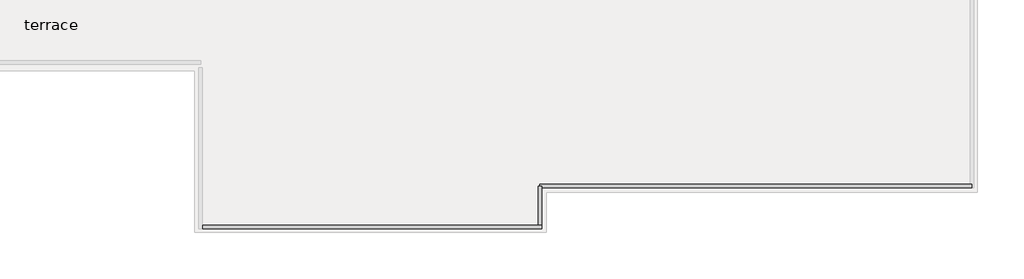
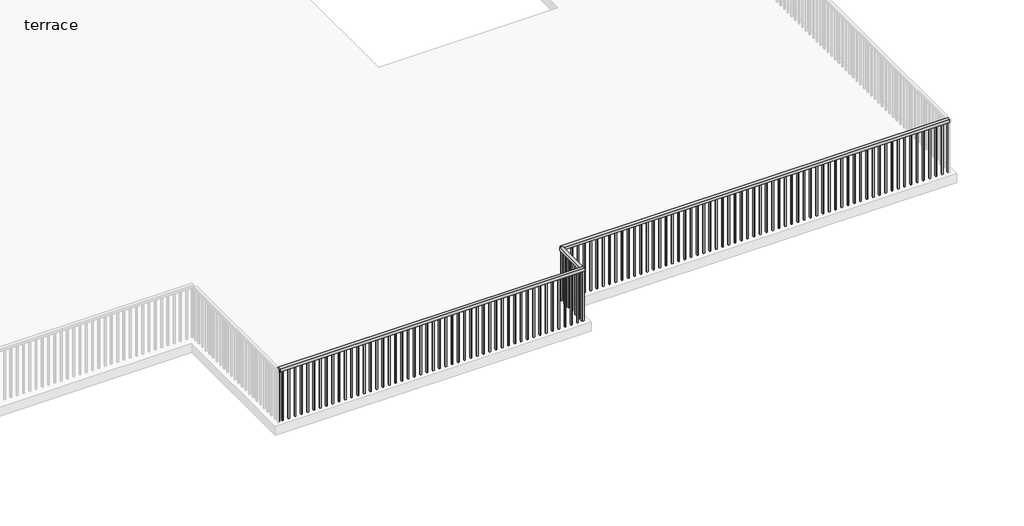
# One storey, part 2 of 7: 3 railings.
"""IFC4 building model written with IfcOpenShell, lengths in millimetres."""

from ifc_helpers import new_model, si_unit, frame, origin, place, context, project, spatial, polyline, outline, extrude, element, save

model = new_model("IFC4")

# Units and contexts
model_context = context("Model", 3, world=origin())
ifc_project = project(units=[si_unit("LENGTHUNIT", "METRE", prefix="MILLI")], contexts=[model_context])

# Site, building, storey
site = spatial("IfcSite", under=ifc_project)
building = spatial("IfcBuilding", under=site)
storey = spatial("IfcBuildingStorey", under=building, Name="terrace", Elevation=3810.0)

# Railings
placement = place(None, origin())
element("IfcRailing", 1, ObjectType="Handrail - Rectangular", at=placement, inside=storey, context=model_context, shape_type="SweptSolid", body=[
    extrude(outline(polyline([(1292.9109871, -4498.672378), (1292.9109871, -4549.472378), (-4974.5390129, -4549.472378), (-4974.5390129, -4498.672378), (1292.9109871, -4498.672378)])), frame((0.0, 0.0, 4673.6), z_axis=(0.0, 0.0, 1.0), x_axis=(1.0, 0.0, 0.0)), (0.0, 0.0, 1.0), 50.8),
    extrude(outline(polyline([(-4895.1640129, -4514.547378), (-4895.1640129, -4533.597378), (-4914.2140129, -4533.597378), (-4914.2140129, -4514.547378), (-4895.1640129, -4514.547378)])), frame((0.0, 0.0, 3810.0), z_axis=(0.0, 0.0, 1.0), x_axis=(1.0, 0.0, 0.0)), (0.0, 0.0, 1.0), 863.6),
    extrude(outline(polyline([(-4793.5640129, -4514.547378), (-4793.5640129, -4533.597378), (-4812.6140129, -4533.597378), (-4812.6140129, -4514.547378), (-4793.5640129, -4514.547378)])), frame((0.0, 0.0, 3810.0), z_axis=(0.0, 0.0, 1.0), x_axis=(1.0, 0.0, 0.0)), (0.0, 0.0, 1.0), 863.6),
    extrude(outline(polyline([(-4691.9640129, -4514.547378), (-4691.9640129, -4533.597378), (-4711.0140129, -4533.597378), (-4711.0140129, -4514.547378), (-4691.9640129, -4514.547378)])), frame((0.0, 0.0, 3810.0), z_axis=(0.0, 0.0, 1.0), x_axis=(1.0, 0.0, 0.0)), (0.0, 0.0, 1.0), 863.6),
    extrude(outline(polyline([(-4590.3640129, -4514.547378), (-4590.3640129, -4533.597378), (-4609.4140129, -4533.597378), (-4609.4140129, -4514.547378), (-4590.3640129, -4514.547378)])), frame((0.0, 0.0, 3810.0), z_axis=(0.0, 0.0, 1.0), x_axis=(1.0, 0.0, 0.0)), (0.0, 0.0, 1.0), 863.6),
    extrude(outline(polyline([(-4488.7640129, -4514.547378), (-4488.7640129, -4533.597378), (-4507.8140129, -4533.597378), (-4507.8140129, -4514.547378), (-4488.7640129, -4514.547378)])), frame((0.0, 0.0, 3810.0), z_axis=(0.0, 0.0, 1.0), x_axis=(1.0, 0.0, 0.0)), (0.0, 0.0, 1.0), 863.6),
    extrude(outline(polyline([(-4387.1640129, -4514.547378), (-4387.1640129, -4533.597378), (-4406.2140129, -4533.597378), (-4406.2140129, -4514.547378), (-4387.1640129, -4514.547378)])), frame((0.0, 0.0, 3810.0), z_axis=(0.0, 0.0, 1.0), x_axis=(1.0, 0.0, 0.0)), (0.0, 0.0, 1.0), 863.6),
    extrude(outline(polyline([(-4285.5640129, -4514.547378), (-4285.5640129, -4533.597378), (-4304.6140129, -4533.597378), (-4304.6140129, -4514.547378), (-4285.5640129, -4514.547378)])), frame((0.0, 0.0, 3810.0), z_axis=(0.0, 0.0, 1.0), x_axis=(1.0, 0.0, 0.0)), (0.0, 0.0, 1.0), 863.6),
    extrude(outline(polyline([(-4183.9640129, -4514.547378), (-4183.9640129, -4533.597378), (-4203.0140129, -4533.597378), (-4203.0140129, -4514.547378), (-4183.9640129, -4514.547378)])), frame((0.0, 0.0, 3810.0), z_axis=(0.0, 0.0, 1.0), x_axis=(1.0, 0.0, 0.0)), (0.0, 0.0, 1.0), 863.6),
    extrude(outline(polyline([(-4082.3640129, -4514.547378), (-4082.3640129, -4533.597378), (-4101.4140129, -4533.597378), (-4101.4140129, -4514.547378), (-4082.3640129, -4514.547378)])), frame((0.0, 0.0, 3810.0), z_axis=(0.0, 0.0, 1.0), x_axis=(1.0, 0.0, 0.0)), (0.0, 0.0, 1.0), 863.6),
    extrude(outline(polyline([(-3980.7640129, -4514.547378), (-3980.7640129, -4533.597378), (-3999.8140129, -4533.597378), (-3999.8140129, -4514.547378), (-3980.7640129, -4514.547378)])), frame((0.0, 0.0, 3810.0), z_axis=(0.0, 0.0, 1.0), x_axis=(1.0, 0.0, 0.0)), (0.0, 0.0, 1.0), 863.6),
    extrude(outline(polyline([(-3879.1640129, -4514.547378), (-3879.1640129, -4533.597378), (-3898.2140129, -4533.597378), (-3898.2140129, -4514.547378), (-3879.1640129, -4514.547378)])), frame((0.0, 0.0, 3810.0), z_axis=(0.0, 0.0, 1.0), x_axis=(1.0, 0.0, 0.0)), (0.0, 0.0, 1.0), 863.6),
    extrude(outline(polyline([(-3777.5640129, -4514.547378), (-3777.5640129, -4533.597378), (-3796.6140129, -4533.597378), (-3796.6140129, -4514.547378), (-3777.5640129, -4514.547378)])), frame((0.0, 0.0, 3810.0), z_axis=(0.0, 0.0, 1.0), x_axis=(1.0, 0.0, 0.0)), (0.0, 0.0, 1.0), 863.6),
    extrude(outline(polyline([(-3675.9640129, -4514.547378), (-3675.9640129, -4533.597378), (-3695.0140129, -4533.597378), (-3695.0140129, -4514.547378), (-3675.9640129, -4514.547378)])), frame((0.0, 0.0, 3810.0), z_axis=(0.0, 0.0, 1.0), x_axis=(1.0, 0.0, 0.0)), (0.0, 0.0, 1.0), 863.6),
    extrude(outline(polyline([(-3574.3640129, -4514.547378), (-3574.3640129, -4533.597378), (-3593.4140129, -4533.597378), (-3593.4140129, -4514.547378), (-3574.3640129, -4514.547378)])), frame((0.0, 0.0, 3810.0), z_axis=(0.0, 0.0, 1.0), x_axis=(1.0, 0.0, 0.0)), (0.0, 0.0, 1.0), 863.6),
    extrude(outline(polyline([(-3472.7640129, -4514.547378), (-3472.7640129, -4533.597378), (-3491.8140129, -4533.597378), (-3491.8140129, -4514.547378), (-3472.7640129, -4514.547378)])), frame((0.0, 0.0, 3810.0), z_axis=(0.0, 0.0, 1.0), x_axis=(1.0, 0.0, 0.0)), (0.0, 0.0, 1.0), 863.6),
    extrude(outline(polyline([(-3371.1640129, -4514.547378), (-3371.1640129, -4533.597378), (-3390.2140129, -4533.597378), (-3390.2140129, -4514.547378), (-3371.1640129, -4514.547378)])), frame((0.0, 0.0, 3810.0), z_axis=(0.0, 0.0, 1.0), x_axis=(1.0, 0.0, 0.0)), (0.0, 0.0, 1.0), 863.6),
    extrude(outline(polyline([(-3269.5640129, -4514.547378), (-3269.5640129, -4533.597378), (-3288.6140129, -4533.597378), (-3288.6140129, -4514.547378), (-3269.5640129, -4514.547378)])), frame((0.0, 0.0, 3810.0), z_axis=(0.0, 0.0, 1.0), x_axis=(1.0, 0.0, 0.0)), (0.0, 0.0, 1.0), 863.6),
    extrude(outline(polyline([(-3167.9640129, -4514.547378), (-3167.9640129, -4533.597378), (-3187.0140129, -4533.597378), (-3187.0140129, -4514.547378), (-3167.9640129, -4514.547378)])), frame((0.0, 0.0, 3810.0), z_axis=(0.0, 0.0, 1.0), x_axis=(1.0, 0.0, 0.0)), (0.0, 0.0, 1.0), 863.6),
    extrude(outline(polyline([(-3066.3640129, -4514.547378), (-3066.3640129, -4533.597378), (-3085.4140129, -4533.597378), (-3085.4140129, -4514.547378), (-3066.3640129, -4514.547378)])), frame((0.0, 0.0, 3810.0), z_axis=(0.0, 0.0, 1.0), x_axis=(1.0, 0.0, 0.0)), (0.0, 0.0, 1.0), 863.6),
    extrude(outline(polyline([(-2964.7640129, -4514.547378), (-2964.7640129, -4533.597378), (-2983.8140129, -4533.597378), (-2983.8140129, -4514.547378), (-2964.7640129, -4514.547378)])), frame((0.0, 0.0, 3810.0), z_axis=(0.0, 0.0, 1.0), x_axis=(1.0, 0.0, 0.0)), (0.0, 0.0, 1.0), 863.6),
    extrude(outline(polyline([(-2863.1640129, -4514.547378), (-2863.1640129, -4533.597378), (-2882.2140129, -4533.597378), (-2882.2140129, -4514.547378), (-2863.1640129, -4514.547378)])), frame((0.0, 0.0, 3810.0), z_axis=(0.0, 0.0, 1.0), x_axis=(1.0, 0.0, 0.0)), (0.0, 0.0, 1.0), 863.6),
    extrude(outline(polyline([(-2761.5640129, -4514.547378), (-2761.5640129, -4533.597378), (-2780.6140129, -4533.597378), (-2780.6140129, -4514.547378), (-2761.5640129, -4514.547378)])), frame((0.0, 0.0, 3810.0), z_axis=(0.0, 0.0, 1.0), x_axis=(1.0, 0.0, 0.0)), (0.0, 0.0, 1.0), 863.6),
    extrude(outline(polyline([(-2659.9640129, -4514.547378), (-2659.9640129, -4533.597378), (-2679.0140129, -4533.597378), (-2679.0140129, -4514.547378), (-2659.9640129, -4514.547378)])), frame((0.0, 0.0, 3810.0), z_axis=(0.0, 0.0, 1.0), x_axis=(1.0, 0.0, 0.0)), (0.0, 0.0, 1.0), 863.6),
    extrude(outline(polyline([(-2558.3640129, -4514.547378), (-2558.3640129, -4533.597378), (-2577.4140129, -4533.597378), (-2577.4140129, -4514.547378), (-2558.3640129, -4514.547378)])), frame((0.0, 0.0, 3810.0), z_axis=(0.0, 0.0, 1.0), x_axis=(1.0, 0.0, 0.0)), (0.0, 0.0, 1.0), 863.6),
    extrude(outline(polyline([(-2456.7640129, -4514.547378), (-2456.7640129, -4533.597378), (-2475.8140129, -4533.597378), (-2475.8140129, -4514.547378), (-2456.7640129, -4514.547378)])), frame((0.0, 0.0, 3810.0), z_axis=(0.0, 0.0, 1.0), x_axis=(1.0, 0.0, 0.0)), (0.0, 0.0, 1.0), 863.6),
    extrude(outline(polyline([(-2355.1640129, -4514.547378), (-2355.1640129, -4533.597378), (-2374.2140129, -4533.597378), (-2374.2140129, -4514.547378), (-2355.1640129, -4514.547378)])), frame((0.0, 0.0, 3810.0), z_axis=(0.0, 0.0, 1.0), x_axis=(1.0, 0.0, 0.0)), (0.0, 0.0, 1.0), 863.6),
    extrude(outline(polyline([(-2253.5640129, -4514.547378), (-2253.5640129, -4533.597378), (-2272.6140129, -4533.597378), (-2272.6140129, -4514.547378), (-2253.5640129, -4514.547378)])), frame((0.0, 0.0, 3810.0), z_axis=(0.0, 0.0, 1.0), x_axis=(1.0, 0.0, 0.0)), (0.0, 0.0, 1.0), 863.6),
    extrude(outline(polyline([(-2151.9640129, -4514.547378), (-2151.9640129, -4533.597378), (-2171.0140129, -4533.597378), (-2171.0140129, -4514.547378), (-2151.9640129, -4514.547378)])), frame((0.0, 0.0, 3810.0), z_axis=(0.0, 0.0, 1.0), x_axis=(1.0, 0.0, 0.0)), (0.0, 0.0, 1.0), 863.6),
    extrude(outline(polyline([(-2050.3640129, -4514.547378), (-2050.3640129, -4533.597378), (-2069.4140129, -4533.597378), (-2069.4140129, -4514.547378), (-2050.3640129, -4514.547378)])), frame((0.0, 0.0, 3810.0), z_axis=(0.0, 0.0, 1.0), x_axis=(1.0, 0.0, 0.0)), (0.0, 0.0, 1.0), 863.6),
    extrude(outline(polyline([(-1948.7640129, -4514.547378), (-1948.7640129, -4533.597378), (-1967.8140129, -4533.597378), (-1967.8140129, -4514.547378), (-1948.7640129, -4514.547378)])), frame((0.0, 0.0, 3810.0), z_axis=(0.0, 0.0, 1.0), x_axis=(1.0, 0.0, 0.0)), (0.0, 0.0, 1.0), 863.6),
    extrude(outline(polyline([(-1847.1640129, -4514.547378), (-1847.1640129, -4533.597378), (-1866.2140129, -4533.597378), (-1866.2140129, -4514.547378), (-1847.1640129, -4514.547378)])), frame((0.0, 0.0, 3810.0), z_axis=(0.0, 0.0, 1.0), x_axis=(1.0, 0.0, 0.0)), (0.0, 0.0, 1.0), 863.6),
    extrude(outline(polyline([(-1745.5640129, -4514.547378), (-1745.5640129, -4533.597378), (-1764.6140129, -4533.597378), (-1764.6140129, -4514.547378), (-1745.5640129, -4514.547378)])), frame((0.0, 0.0, 3810.0), z_axis=(0.0, 0.0, 1.0), x_axis=(1.0, 0.0, 0.0)), (0.0, 0.0, 1.0), 863.6),
    extrude(outline(polyline([(-1643.9640129, -4514.547378), (-1643.9640129, -4533.597378), (-1663.0140129, -4533.597378), (-1663.0140129, -4514.547378), (-1643.9640129, -4514.547378)])), frame((0.0, 0.0, 3810.0), z_axis=(0.0, 0.0, 1.0), x_axis=(1.0, 0.0, 0.0)), (0.0, 0.0, 1.0), 863.6),
    extrude(outline(polyline([(-1542.3640129, -4514.547378), (-1542.3640129, -4533.597378), (-1561.4140129, -4533.597378), (-1561.4140129, -4514.547378), (-1542.3640129, -4514.547378)])), frame((0.0, 0.0, 3810.0), z_axis=(0.0, 0.0, 1.0), x_axis=(1.0, 0.0, 0.0)), (0.0, 0.0, 1.0), 863.6),
    extrude(outline(polyline([(-1440.7640129, -4514.547378), (-1440.7640129, -4533.597378), (-1459.8140129, -4533.597378), (-1459.8140129, -4514.547378), (-1440.7640129, -4514.547378)])), frame((0.0, 0.0, 3810.0), z_axis=(0.0, 0.0, 1.0), x_axis=(1.0, 0.0, 0.0)), (0.0, 0.0, 1.0), 863.6),
    extrude(outline(polyline([(-1339.1640129, -4514.547378), (-1339.1640129, -4533.597378), (-1358.2140129, -4533.597378), (-1358.2140129, -4514.547378), (-1339.1640129, -4514.547378)])), frame((0.0, 0.0, 3810.0), z_axis=(0.0, 0.0, 1.0), x_axis=(1.0, 0.0, 0.0)), (0.0, 0.0, 1.0), 863.6),
    extrude(outline(polyline([(-1237.5640129, -4514.547378), (-1237.5640129, -4533.597378), (-1256.6140129, -4533.597378), (-1256.6140129, -4514.547378), (-1237.5640129, -4514.547378)])), frame((0.0, 0.0, 3810.0), z_axis=(0.0, 0.0, 1.0), x_axis=(1.0, 0.0, 0.0)), (0.0, 0.0, 1.0), 863.6),
    extrude(outline(polyline([(-1135.9640129, -4514.547378), (-1135.9640129, -4533.597378), (-1155.0140129, -4533.597378), (-1155.0140129, -4514.547378), (-1135.9640129, -4514.547378)])), frame((0.0, 0.0, 3810.0), z_axis=(0.0, 0.0, 1.0), x_axis=(1.0, 0.0, 0.0)), (0.0, 0.0, 1.0), 863.6),
    extrude(outline(polyline([(-1034.3640129, -4514.547378), (-1034.3640129, -4533.597378), (-1053.4140129, -4533.597378), (-1053.4140129, -4514.547378), (-1034.3640129, -4514.547378)])), frame((0.0, 0.0, 3810.0), z_axis=(0.0, 0.0, 1.0), x_axis=(1.0, 0.0, 0.0)), (0.0, 0.0, 1.0), 863.6),
    extrude(outline(polyline([(-932.7640129, -4514.547378), (-932.7640129, -4533.597378), (-951.8140129, -4533.597378), (-951.8140129, -4514.547378), (-932.7640129, -4514.547378)])), frame((0.0, 0.0, 3810.0), z_axis=(0.0, 0.0, 1.0), x_axis=(1.0, 0.0, 0.0)), (0.0, 0.0, 1.0), 863.6),
    extrude(outline(polyline([(-831.1640129, -4514.547378), (-831.1640129, -4533.597378), (-850.2140129, -4533.597378), (-850.2140129, -4514.547378), (-831.1640129, -4514.547378)])), frame((0.0, 0.0, 3810.0), z_axis=(0.0, 0.0, 1.0), x_axis=(1.0, 0.0, 0.0)), (0.0, 0.0, 1.0), 863.6),
    extrude(outline(polyline([(-729.5640129, -4514.547378), (-729.5640129, -4533.597378), (-748.6140129, -4533.597378), (-748.6140129, -4514.547378), (-729.5640129, -4514.547378)])), frame((0.0, 0.0, 3810.0), z_axis=(0.0, 0.0, 1.0), x_axis=(1.0, 0.0, 0.0)), (0.0, 0.0, 1.0), 863.6),
    extrude(outline(polyline([(-627.9640129, -4514.547378), (-627.9640129, -4533.597378), (-647.0140129, -4533.597378), (-647.0140129, -4514.547378), (-627.9640129, -4514.547378)])), frame((0.0, 0.0, 3810.0), z_axis=(0.0, 0.0, 1.0), x_axis=(1.0, 0.0, 0.0)), (0.0, 0.0, 1.0), 863.6),
    extrude(outline(polyline([(-526.3640129, -4514.547378), (-526.3640129, -4533.597378), (-545.4140129, -4533.597378), (-545.4140129, -4514.547378), (-526.3640129, -4514.547378)])), frame((0.0, 0.0, 3810.0), z_axis=(0.0, 0.0, 1.0), x_axis=(1.0, 0.0, 0.0)), (0.0, 0.0, 1.0), 863.6),
    extrude(outline(polyline([(-424.7640129, -4514.547378), (-424.7640129, -4533.597378), (-443.8140129, -4533.597378), (-443.8140129, -4514.547378), (-424.7640129, -4514.547378)])), frame((0.0, 0.0, 3810.0), z_axis=(0.0, 0.0, 1.0), x_axis=(1.0, 0.0, 0.0)), (0.0, 0.0, 1.0), 863.6),
    extrude(outline(polyline([(-323.1640129, -4514.547378), (-323.1640129, -4533.597378), (-342.2140129, -4533.597378), (-342.2140129, -4514.547378), (-323.1640129, -4514.547378)])), frame((0.0, 0.0, 3810.0), z_axis=(0.0, 0.0, 1.0), x_axis=(1.0, 0.0, 0.0)), (0.0, 0.0, 1.0), 863.6),
    extrude(outline(polyline([(-221.5640129, -4514.547378), (-221.5640129, -4533.597378), (-240.6140129, -4533.597378), (-240.6140129, -4514.547378), (-221.5640129, -4514.547378)])), frame((0.0, 0.0, 3810.0), z_axis=(0.0, 0.0, 1.0), x_axis=(1.0, 0.0, 0.0)), (0.0, 0.0, 1.0), 863.6),
    extrude(outline(polyline([(-119.9640129, -4514.547378), (-119.9640129, -4533.597378), (-139.0140129, -4533.597378), (-139.0140129, -4514.547378), (-119.9640129, -4514.547378)])), frame((0.0, 0.0, 3810.0), z_axis=(0.0, 0.0, 1.0), x_axis=(1.0, 0.0, 0.0)), (0.0, 0.0, 1.0), 863.6),
    extrude(outline(polyline([(-18.3640129, -4514.547378), (-18.3640129, -4533.597378), (-37.4140129, -4533.597378), (-37.4140129, -4514.547378), (-18.3640129, -4514.547378)])), frame((0.0, 0.0, 3810.0), z_axis=(0.0, 0.0, 1.0), x_axis=(1.0, 0.0, 0.0)), (0.0, 0.0, 1.0), 863.6),
    extrude(outline(polyline([(83.2359871, -4514.547378), (83.2359871, -4533.597378), (64.1859871, -4533.597378), (64.1859871, -4514.547378), (83.2359871, -4514.547378)])), frame((0.0, 0.0, 3810.0), z_axis=(0.0, 0.0, 1.0), x_axis=(1.0, 0.0, 0.0)), (0.0, 0.0, 1.0), 863.6),
    extrude(outline(polyline([(184.8359871, -4514.547378), (184.8359871, -4533.597378), (165.7859871, -4533.597378), (165.7859871, -4514.547378), (184.8359871, -4514.547378)])), frame((0.0, 0.0, 3810.0), z_axis=(0.0, 0.0, 1.0), x_axis=(1.0, 0.0, 0.0)), (0.0, 0.0, 1.0), 863.6),
    extrude(outline(polyline([(286.4359871, -4514.547378), (286.4359871, -4533.597378), (267.3859871, -4533.597378), (267.3859871, -4514.547378), (286.4359871, -4514.547378)])), frame((0.0, 0.0, 3810.0), z_axis=(0.0, 0.0, 1.0), x_axis=(1.0, 0.0, 0.0)), (0.0, 0.0, 1.0), 863.6),
    extrude(outline(polyline([(388.0359871, -4514.547378), (388.0359871, -4533.597378), (368.9859871, -4533.597378), (368.9859871, -4514.547378), (388.0359871, -4514.547378)])), frame((0.0, 0.0, 3810.0), z_axis=(0.0, 0.0, 1.0), x_axis=(1.0, 0.0, 0.0)), (0.0, 0.0, 1.0), 863.6),
    extrude(outline(polyline([(489.6359871, -4514.547378), (489.6359871, -4533.597378), (470.5859871, -4533.597378), (470.5859871, -4514.547378), (489.6359871, -4514.547378)])), frame((0.0, 0.0, 3810.0), z_axis=(0.0, 0.0, 1.0), x_axis=(1.0, 0.0, 0.0)), (0.0, 0.0, 1.0), 863.6),
    extrude(outline(polyline([(591.2359871, -4514.547378), (591.2359871, -4533.597378), (572.1859871, -4533.597378), (572.1859871, -4514.547378), (591.2359871, -4514.547378)])), frame((0.0, 0.0, 3810.0), z_axis=(0.0, 0.0, 1.0), x_axis=(1.0, 0.0, 0.0)), (0.0, 0.0, 1.0), 863.6),
    extrude(outline(polyline([(692.8359871, -4514.547378), (692.8359871, -4533.597378), (673.7859871, -4533.597378), (673.7859871, -4514.547378), (692.8359871, -4514.547378)])), frame((0.0, 0.0, 3810.0), z_axis=(0.0, 0.0, 1.0), x_axis=(1.0, 0.0, 0.0)), (0.0, 0.0, 1.0), 863.6),
    extrude(outline(polyline([(794.4359871, -4514.547378), (794.4359871, -4533.597378), (775.3859871, -4533.597378), (775.3859871, -4514.547378), (794.4359871, -4514.547378)])), frame((0.0, 0.0, 3810.0), z_axis=(0.0, 0.0, 1.0), x_axis=(1.0, 0.0, 0.0)), (0.0, 0.0, 1.0), 863.6),
    extrude(outline(polyline([(896.0359871, -4514.547378), (896.0359871, -4533.597378), (876.9859871, -4533.597378), (876.9859871, -4514.547378), (896.0359871, -4514.547378)])), frame((0.0, 0.0, 3810.0), z_axis=(0.0, 0.0, 1.0), x_axis=(1.0, 0.0, 0.0)), (0.0, 0.0, 1.0), 863.6),
    extrude(outline(polyline([(997.6359871, -4514.547378), (997.6359871, -4533.597378), (978.5859871, -4533.597378), (978.5859871, -4514.547378), (997.6359871, -4514.547378)])), frame((0.0, 0.0, 3810.0), z_axis=(0.0, 0.0, 1.0), x_axis=(1.0, 0.0, 0.0)), (0.0, 0.0, 1.0), 863.6),
    extrude(outline(polyline([(1099.2359871, -4514.547378), (1099.2359871, -4533.597378), (1080.1859871, -4533.597378), (1080.1859871, -4514.547378), (1099.2359871, -4514.547378)])), frame((0.0, 0.0, 3810.0), z_axis=(0.0, 0.0, 1.0), x_axis=(1.0, 0.0, 0.0)), (0.0, 0.0, 1.0), 863.6),
    extrude(outline(polyline([(1200.8359871, -4514.547378), (1200.8359871, -4533.597378), (1181.7859871, -4533.597378), (1181.7859871, -4514.547378), (1200.8359871, -4514.547378)])), frame((0.0, 0.0, 3810.0), z_axis=(0.0, 0.0, 1.0), x_axis=(1.0, 0.0, 0.0)), (0.0, 0.0, 1.0), 863.6),
    extrude(outline(polyline([(-4955.4890129, -4514.547378), (-4955.4890129, -4533.597378), (-4974.5390129, -4533.597378), (-4974.5390129, -4514.547378), (-4955.4890129, -4514.547378)])), frame((0.0, 0.0, 3810.0), z_axis=(0.0, 0.0, 1.0), x_axis=(1.0, 0.0, 0.0)), (0.0, 0.0, 1.0), 863.6),
    extrude(outline(polyline([(1292.9109871, -4514.547378), (1292.9109871, -4533.597378), (1273.8609871, -4533.597378), (1273.8609871, -4514.547378), (1292.9109871, -4514.547378)])), frame((0.0, 0.0, 3810.0), z_axis=(0.0, 0.0, 1.0), x_axis=(1.0, 0.0, 0.0)), (0.0, 0.0, 1.0), 863.6),
])
element("IfcRailing", 2, ObjectType="Handrail - Rectangular", at=placement, inside=storey, context=model_context, shape_type="SweptSolid", body=[
    extrude(outline(polyline([(-4999.9390129, -4524.072378), (-4949.1390129, -4524.072378), (-4949.1390129, -5114.622378), (-4999.9390129, -5114.622378), (-4999.9390129, -4524.072378)])), frame((0.0, 0.0, 4673.6), z_axis=(0.0, 0.0, 1.0), x_axis=(1.0, 0.0, 0.0)), (0.0, 0.0, 1.0), 50.8),
    extrude(outline(polyline([(-4984.0640129, -5022.547378), (-4965.0140129, -5022.547378), (-4965.0140129, -5041.597378), (-4984.0640129, -5041.597378), (-4984.0640129, -5022.547378)])), frame((0.0, 0.0, 3810.0), z_axis=(0.0, 0.0, 1.0), x_axis=(1.0, 0.0, 0.0)), (0.0, 0.0, 1.0), 863.6),
    extrude(outline(polyline([(-4984.0640129, -4920.947378), (-4965.0140129, -4920.947378), (-4965.0140129, -4939.997378), (-4984.0640129, -4939.997378), (-4984.0640129, -4920.947378)])), frame((0.0, 0.0, 3810.0), z_axis=(0.0, 0.0, 1.0), x_axis=(1.0, 0.0, 0.0)), (0.0, 0.0, 1.0), 863.6),
    extrude(outline(polyline([(-4984.0640129, -4819.347378), (-4965.0140129, -4819.347378), (-4965.0140129, -4838.397378), (-4984.0640129, -4838.397378), (-4984.0640129, -4819.347378)])), frame((0.0, 0.0, 3810.0), z_axis=(0.0, 0.0, 1.0), x_axis=(1.0, 0.0, 0.0)), (0.0, 0.0, 1.0), 863.6),
    extrude(outline(polyline([(-4984.0640129, -4717.747378), (-4965.0140129, -4717.747378), (-4965.0140129, -4736.797378), (-4984.0640129, -4736.797378), (-4984.0640129, -4717.747378)])), frame((0.0, 0.0, 3810.0), z_axis=(0.0, 0.0, 1.0), x_axis=(1.0, 0.0, 0.0)), (0.0, 0.0, 1.0), 863.6),
    extrude(outline(polyline([(-4984.0640129, -4616.147378), (-4965.0140129, -4616.147378), (-4965.0140129, -4635.197378), (-4984.0640129, -4635.197378), (-4984.0640129, -4616.147378)])), frame((0.0, 0.0, 3810.0), z_axis=(0.0, 0.0, 1.0), x_axis=(1.0, 0.0, 0.0)), (0.0, 0.0, 1.0), 863.6),
    extrude(outline(polyline([(-4984.0640129, -5095.572378), (-4965.0140129, -5095.572378), (-4965.0140129, -5114.622378), (-4984.0640129, -5114.622378), (-4984.0640129, -5095.572378)])), frame((0.0, 0.0, 3810.0), z_axis=(0.0, 0.0, 1.0), x_axis=(1.0, 0.0, 0.0)), (0.0, 0.0, 1.0), 863.6),
    extrude(outline(polyline([(-4984.0640129, -4524.072378), (-4965.0140129, -4524.072378), (-4965.0140129, -4543.122378), (-4984.0640129, -4543.122378), (-4984.0640129, -4524.072378)])), frame((0.0, 0.0, 3810.0), z_axis=(0.0, 0.0, 1.0), x_axis=(1.0, 0.0, 0.0)), (0.0, 0.0, 1.0), 863.6),
])
element("IfcRailing", 3, ObjectType="Handrail - Rectangular", at=placement, inside=storey, context=model_context, shape_type="SweptSolid", body=[
    extrude(outline(polyline([(-4949.1390129, -5089.222378), (-4949.1390129, -5140.022378), (-9895.7890129, -5140.022378), (-9895.7890129, -5089.222378), (-4949.1390129, -5089.222378)])), frame((0.0, 0.0, 4673.6), z_axis=(0.0, 0.0, 1.0), x_axis=(1.0, 0.0, 0.0)), (0.0, 0.0, 1.0), 50.8),
    extrude(outline(polyline([(-9816.4140129, -5105.097378), (-9816.4140129, -5124.147378), (-9835.4640129, -5124.147378), (-9835.4640129, -5105.097378), (-9816.4140129, -5105.097378)])), frame((0.0, 0.0, 3810.0), z_axis=(0.0, 0.0, 1.0), x_axis=(1.0, 0.0, 0.0)), (0.0, 0.0, 1.0), 863.6),
    extrude(outline(polyline([(-9714.8140129, -5105.097378), (-9714.8140129, -5124.147378), (-9733.8640129, -5124.147378), (-9733.8640129, -5105.097378), (-9714.8140129, -5105.097378)])), frame((0.0, 0.0, 3810.0), z_axis=(0.0, 0.0, 1.0), x_axis=(1.0, 0.0, 0.0)), (0.0, 0.0, 1.0), 863.6),
    extrude(outline(polyline([(-9613.2140129, -5105.097378), (-9613.2140129, -5124.147378), (-9632.2640129, -5124.147378), (-9632.2640129, -5105.097378), (-9613.2140129, -5105.097378)])), frame((0.0, 0.0, 3810.0), z_axis=(0.0, 0.0, 1.0), x_axis=(1.0, 0.0, 0.0)), (0.0, 0.0, 1.0), 863.6),
    extrude(outline(polyline([(-9511.6140129, -5105.097378), (-9511.6140129, -5124.147378), (-9530.6640129, -5124.147378), (-9530.6640129, -5105.097378), (-9511.6140129, -5105.097378)])), frame((0.0, 0.0, 3810.0), z_axis=(0.0, 0.0, 1.0), x_axis=(1.0, 0.0, 0.0)), (0.0, 0.0, 1.0), 863.6),
    extrude(outline(polyline([(-9410.0140129, -5105.097378), (-9410.0140129, -5124.147378), (-9429.0640129, -5124.147378), (-9429.0640129, -5105.097378), (-9410.0140129, -5105.097378)])), frame((0.0, 0.0, 3810.0), z_axis=(0.0, 0.0, 1.0), x_axis=(1.0, 0.0, 0.0)), (0.0, 0.0, 1.0), 863.6),
    extrude(outline(polyline([(-9308.4140129, -5105.097378), (-9308.4140129, -5124.147378), (-9327.4640129, -5124.147378), (-9327.4640129, -5105.097378), (-9308.4140129, -5105.097378)])), frame((0.0, 0.0, 3810.0), z_axis=(0.0, 0.0, 1.0), x_axis=(1.0, 0.0, 0.0)), (0.0, 0.0, 1.0), 863.6),
    extrude(outline(polyline([(-9206.8140129, -5105.097378), (-9206.8140129, -5124.147378), (-9225.8640129, -5124.147378), (-9225.8640129, -5105.097378), (-9206.8140129, -5105.097378)])), frame((0.0, 0.0, 3810.0), z_axis=(0.0, 0.0, 1.0), x_axis=(1.0, 0.0, 0.0)), (0.0, 0.0, 1.0), 863.6),
    extrude(outline(polyline([(-9105.2140129, -5105.097378), (-9105.2140129, -5124.147378), (-9124.2640129, -5124.147378), (-9124.2640129, -5105.097378), (-9105.2140129, -5105.097378)])), frame((0.0, 0.0, 3810.0), z_axis=(0.0, 0.0, 1.0), x_axis=(1.0, 0.0, 0.0)), (0.0, 0.0, 1.0), 863.6),
    extrude(outline(polyline([(-9003.6140129, -5105.097378), (-9003.6140129, -5124.147378), (-9022.6640129, -5124.147378), (-9022.6640129, -5105.097378), (-9003.6140129, -5105.097378)])), frame((0.0, 0.0, 3810.0), z_axis=(0.0, 0.0, 1.0), x_axis=(1.0, 0.0, 0.0)), (0.0, 0.0, 1.0), 863.6),
    extrude(outline(polyline([(-8902.0140129, -5105.097378), (-8902.0140129, -5124.147378), (-8921.0640129, -5124.147378), (-8921.0640129, -5105.097378), (-8902.0140129, -5105.097378)])), frame((0.0, 0.0, 3810.0), z_axis=(0.0, 0.0, 1.0), x_axis=(1.0, 0.0, 0.0)), (0.0, 0.0, 1.0), 863.6),
    extrude(outline(polyline([(-8800.4140129, -5105.097378), (-8800.4140129, -5124.147378), (-8819.4640129, -5124.147378), (-8819.4640129, -5105.097378), (-8800.4140129, -5105.097378)])), frame((0.0, 0.0, 3810.0), z_axis=(0.0, 0.0, 1.0), x_axis=(1.0, 0.0, 0.0)), (0.0, 0.0, 1.0), 863.6),
    extrude(outline(polyline([(-8698.8140129, -5105.097378), (-8698.8140129, -5124.147378), (-8717.8640129, -5124.147378), (-8717.8640129, -5105.097378), (-8698.8140129, -5105.097378)])), frame((0.0, 0.0, 3810.0), z_axis=(0.0, 0.0, 1.0), x_axis=(1.0, 0.0, 0.0)), (0.0, 0.0, 1.0), 863.6),
    extrude(outline(polyline([(-8597.2140129, -5105.097378), (-8597.2140129, -5124.147378), (-8616.2640129, -5124.147378), (-8616.2640129, -5105.097378), (-8597.2140129, -5105.097378)])), frame((0.0, 0.0, 3810.0), z_axis=(0.0, 0.0, 1.0), x_axis=(1.0, 0.0, 0.0)), (0.0, 0.0, 1.0), 863.6),
    extrude(outline(polyline([(-8495.6140129, -5105.097378), (-8495.6140129, -5124.147378), (-8514.6640129, -5124.147378), (-8514.6640129, -5105.097378), (-8495.6140129, -5105.097378)])), frame((0.0, 0.0, 3810.0), z_axis=(0.0, 0.0, 1.0), x_axis=(1.0, 0.0, 0.0)), (0.0, 0.0, 1.0), 863.6),
    extrude(outline(polyline([(-8394.0140129, -5105.097378), (-8394.0140129, -5124.147378), (-8413.0640129, -5124.147378), (-8413.0640129, -5105.097378), (-8394.0140129, -5105.097378)])), frame((0.0, 0.0, 3810.0), z_axis=(0.0, 0.0, 1.0), x_axis=(1.0, 0.0, 0.0)), (0.0, 0.0, 1.0), 863.6),
    extrude(outline(polyline([(-8292.4140129, -5105.097378), (-8292.4140129, -5124.147378), (-8311.4640129, -5124.147378), (-8311.4640129, -5105.097378), (-8292.4140129, -5105.097378)])), frame((0.0, 0.0, 3810.0), z_axis=(0.0, 0.0, 1.0), x_axis=(1.0, 0.0, 0.0)), (0.0, 0.0, 1.0), 863.6),
    extrude(outline(polyline([(-8190.8140129, -5105.097378), (-8190.8140129, -5124.147378), (-8209.8640129, -5124.147378), (-8209.8640129, -5105.097378), (-8190.8140129, -5105.097378)])), frame((0.0, 0.0, 3810.0), z_axis=(0.0, 0.0, 1.0), x_axis=(1.0, 0.0, 0.0)), (0.0, 0.0, 1.0), 863.6),
    extrude(outline(polyline([(-8089.2140129, -5105.097378), (-8089.2140129, -5124.147378), (-8108.2640129, -5124.147378), (-8108.2640129, -5105.097378), (-8089.2140129, -5105.097378)])), frame((0.0, 0.0, 3810.0), z_axis=(0.0, 0.0, 1.0), x_axis=(1.0, 0.0, 0.0)), (0.0, 0.0, 1.0), 863.6),
    extrude(outline(polyline([(-7987.6140129, -5105.097378), (-7987.6140129, -5124.147378), (-8006.6640129, -5124.147378), (-8006.6640129, -5105.097378), (-7987.6140129, -5105.097378)])), frame((0.0, 0.0, 3810.0), z_axis=(0.0, 0.0, 1.0), x_axis=(1.0, 0.0, 0.0)), (0.0, 0.0, 1.0), 863.6),
    extrude(outline(polyline([(-7886.0140129, -5105.097378), (-7886.0140129, -5124.147378), (-7905.0640129, -5124.147378), (-7905.0640129, -5105.097378), (-7886.0140129, -5105.097378)])), frame((0.0, 0.0, 3810.0), z_axis=(0.0, 0.0, 1.0), x_axis=(1.0, 0.0, 0.0)), (0.0, 0.0, 1.0), 863.6),
    extrude(outline(polyline([(-7784.4140129, -5105.097378), (-7784.4140129, -5124.147378), (-7803.4640129, -5124.147378), (-7803.4640129, -5105.097378), (-7784.4140129, -5105.097378)])), frame((0.0, 0.0, 3810.0), z_axis=(0.0, 0.0, 1.0), x_axis=(1.0, 0.0, 0.0)), (0.0, 0.0, 1.0), 863.6),
    extrude(outline(polyline([(-7682.8140129, -5105.097378), (-7682.8140129, -5124.147378), (-7701.8640129, -5124.147378), (-7701.8640129, -5105.097378), (-7682.8140129, -5105.097378)])), frame((0.0, 0.0, 3810.0), z_axis=(0.0, 0.0, 1.0), x_axis=(1.0, 0.0, 0.0)), (0.0, 0.0, 1.0), 863.6),
    extrude(outline(polyline([(-7581.2140129, -5105.097378), (-7581.2140129, -5124.147378), (-7600.2640129, -5124.147378), (-7600.2640129, -5105.097378), (-7581.2140129, -5105.097378)])), frame((0.0, 0.0, 3810.0), z_axis=(0.0, 0.0, 1.0), x_axis=(1.0, 0.0, 0.0)), (0.0, 0.0, 1.0), 863.6),
    extrude(outline(polyline([(-7479.6140129, -5105.097378), (-7479.6140129, -5124.147378), (-7498.6640129, -5124.147378), (-7498.6640129, -5105.097378), (-7479.6140129, -5105.097378)])), frame((0.0, 0.0, 3810.0), z_axis=(0.0, 0.0, 1.0), x_axis=(1.0, 0.0, 0.0)), (0.0, 0.0, 1.0), 863.6),
    extrude(outline(polyline([(-7378.0140129, -5105.097378), (-7378.0140129, -5124.147378), (-7397.0640129, -5124.147378), (-7397.0640129, -5105.097378), (-7378.0140129, -5105.097378)])), frame((0.0, 0.0, 3810.0), z_axis=(0.0, 0.0, 1.0), x_axis=(1.0, 0.0, 0.0)), (0.0, 0.0, 1.0), 863.6),
    extrude(outline(polyline([(-7276.4140129, -5105.097378), (-7276.4140129, -5124.147378), (-7295.4640129, -5124.147378), (-7295.4640129, -5105.097378), (-7276.4140129, -5105.097378)])), frame((0.0, 0.0, 3810.0), z_axis=(0.0, 0.0, 1.0), x_axis=(1.0, 0.0, 0.0)), (0.0, 0.0, 1.0), 863.6),
    extrude(outline(polyline([(-7174.8140129, -5105.097378), (-7174.8140129, -5124.147378), (-7193.8640129, -5124.147378), (-7193.8640129, -5105.097378), (-7174.8140129, -5105.097378)])), frame((0.0, 0.0, 3810.0), z_axis=(0.0, 0.0, 1.0), x_axis=(1.0, 0.0, 0.0)), (0.0, 0.0, 1.0), 863.6),
    extrude(outline(polyline([(-7073.2140129, -5105.097378), (-7073.2140129, -5124.147378), (-7092.2640129, -5124.147378), (-7092.2640129, -5105.097378), (-7073.2140129, -5105.097378)])), frame((0.0, 0.0, 3810.0), z_axis=(0.0, 0.0, 1.0), x_axis=(1.0, 0.0, 0.0)), (0.0, 0.0, 1.0), 863.6),
    extrude(outline(polyline([(-6971.6140129, -5105.097378), (-6971.6140129, -5124.147378), (-6990.6640129, -5124.147378), (-6990.6640129, -5105.097378), (-6971.6140129, -5105.097378)])), frame((0.0, 0.0, 3810.0), z_axis=(0.0, 0.0, 1.0), x_axis=(1.0, 0.0, 0.0)), (0.0, 0.0, 1.0), 863.6),
    extrude(outline(polyline([(-6870.0140129, -5105.097378), (-6870.0140129, -5124.147378), (-6889.0640129, -5124.147378), (-6889.0640129, -5105.097378), (-6870.0140129, -5105.097378)])), frame((0.0, 0.0, 3810.0), z_axis=(0.0, 0.0, 1.0), x_axis=(1.0, 0.0, 0.0)), (0.0, 0.0, 1.0), 863.6),
    extrude(outline(polyline([(-6768.4140129, -5105.097378), (-6768.4140129, -5124.147378), (-6787.4640129, -5124.147378), (-6787.4640129, -5105.097378), (-6768.4140129, -5105.097378)])), frame((0.0, 0.0, 3810.0), z_axis=(0.0, 0.0, 1.0), x_axis=(1.0, 0.0, 0.0)), (0.0, 0.0, 1.0), 863.6),
    extrude(outline(polyline([(-6666.8140129, -5105.097378), (-6666.8140129, -5124.147378), (-6685.8640129, -5124.147378), (-6685.8640129, -5105.097378), (-6666.8140129, -5105.097378)])), frame((0.0, 0.0, 3810.0), z_axis=(0.0, 0.0, 1.0), x_axis=(1.0, 0.0, 0.0)), (0.0, 0.0, 1.0), 863.6),
    extrude(outline(polyline([(-6565.2140129, -5105.097378), (-6565.2140129, -5124.147378), (-6584.2640129, -5124.147378), (-6584.2640129, -5105.097378), (-6565.2140129, -5105.097378)])), frame((0.0, 0.0, 3810.0), z_axis=(0.0, 0.0, 1.0), x_axis=(1.0, 0.0, 0.0)), (0.0, 0.0, 1.0), 863.6),
    extrude(outline(polyline([(-6463.6140129, -5105.097378), (-6463.6140129, -5124.147378), (-6482.6640129, -5124.147378), (-6482.6640129, -5105.097378), (-6463.6140129, -5105.097378)])), frame((0.0, 0.0, 3810.0), z_axis=(0.0, 0.0, 1.0), x_axis=(1.0, 0.0, 0.0)), (0.0, 0.0, 1.0), 863.6),
    extrude(outline(polyline([(-6362.0140129, -5105.097378), (-6362.0140129, -5124.147378), (-6381.0640129, -5124.147378), (-6381.0640129, -5105.097378), (-6362.0140129, -5105.097378)])), frame((0.0, 0.0, 3810.0), z_axis=(0.0, 0.0, 1.0), x_axis=(1.0, 0.0, 0.0)), (0.0, 0.0, 1.0), 863.6),
    extrude(outline(polyline([(-6260.4140129, -5105.097378), (-6260.4140129, -5124.147378), (-6279.4640129, -5124.147378), (-6279.4640129, -5105.097378), (-6260.4140129, -5105.097378)])), frame((0.0, 0.0, 3810.0), z_axis=(0.0, 0.0, 1.0), x_axis=(1.0, 0.0, 0.0)), (0.0, 0.0, 1.0), 863.6),
    extrude(outline(polyline([(-6158.8140129, -5105.097378), (-6158.8140129, -5124.147378), (-6177.8640129, -5124.147378), (-6177.8640129, -5105.097378), (-6158.8140129, -5105.097378)])), frame((0.0, 0.0, 3810.0), z_axis=(0.0, 0.0, 1.0), x_axis=(1.0, 0.0, 0.0)), (0.0, 0.0, 1.0), 863.6),
    extrude(outline(polyline([(-6057.2140129, -5105.097378), (-6057.2140129, -5124.147378), (-6076.2640129, -5124.147378), (-6076.2640129, -5105.097378), (-6057.2140129, -5105.097378)])), frame((0.0, 0.0, 3810.0), z_axis=(0.0, 0.0, 1.0), x_axis=(1.0, 0.0, 0.0)), (0.0, 0.0, 1.0), 863.6),
    extrude(outline(polyline([(-5955.6140129, -5105.097378), (-5955.6140129, -5124.147378), (-5974.6640129, -5124.147378), (-5974.6640129, -5105.097378), (-5955.6140129, -5105.097378)])), frame((0.0, 0.0, 3810.0), z_axis=(0.0, 0.0, 1.0), x_axis=(1.0, 0.0, 0.0)), (0.0, 0.0, 1.0), 863.6),
    extrude(outline(polyline([(-5854.0140129, -5105.097378), (-5854.0140129, -5124.147378), (-5873.0640129, -5124.147378), (-5873.0640129, -5105.097378), (-5854.0140129, -5105.097378)])), frame((0.0, 0.0, 3810.0), z_axis=(0.0, 0.0, 1.0), x_axis=(1.0, 0.0, 0.0)), (0.0, 0.0, 1.0), 863.6),
    extrude(outline(polyline([(-5752.4140129, -5105.097378), (-5752.4140129, -5124.147378), (-5771.4640129, -5124.147378), (-5771.4640129, -5105.097378), (-5752.4140129, -5105.097378)])), frame((0.0, 0.0, 3810.0), z_axis=(0.0, 0.0, 1.0), x_axis=(1.0, 0.0, 0.0)), (0.0, 0.0, 1.0), 863.6),
    extrude(outline(polyline([(-5650.8140129, -5105.097378), (-5650.8140129, -5124.147378), (-5669.8640129, -5124.147378), (-5669.8640129, -5105.097378), (-5650.8140129, -5105.097378)])), frame((0.0, 0.0, 3810.0), z_axis=(0.0, 0.0, 1.0), x_axis=(1.0, 0.0, 0.0)), (0.0, 0.0, 1.0), 863.6),
    extrude(outline(polyline([(-5549.2140129, -5105.097378), (-5549.2140129, -5124.147378), (-5568.2640129, -5124.147378), (-5568.2640129, -5105.097378), (-5549.2140129, -5105.097378)])), frame((0.0, 0.0, 3810.0), z_axis=(0.0, 0.0, 1.0), x_axis=(1.0, 0.0, 0.0)), (0.0, 0.0, 1.0), 863.6),
    extrude(outline(polyline([(-5447.6140129, -5105.097378), (-5447.6140129, -5124.147378), (-5466.6640129, -5124.147378), (-5466.6640129, -5105.097378), (-5447.6140129, -5105.097378)])), frame((0.0, 0.0, 3810.0), z_axis=(0.0, 0.0, 1.0), x_axis=(1.0, 0.0, 0.0)), (0.0, 0.0, 1.0), 863.6),
    extrude(outline(polyline([(-5346.0140129, -5105.097378), (-5346.0140129, -5124.147378), (-5365.0640129, -5124.147378), (-5365.0640129, -5105.097378), (-5346.0140129, -5105.097378)])), frame((0.0, 0.0, 3810.0), z_axis=(0.0, 0.0, 1.0), x_axis=(1.0, 0.0, 0.0)), (0.0, 0.0, 1.0), 863.6),
    extrude(outline(polyline([(-5244.4140129, -5105.097378), (-5244.4140129, -5124.147378), (-5263.4640129, -5124.147378), (-5263.4640129, -5105.097378), (-5244.4140129, -5105.097378)])), frame((0.0, 0.0, 3810.0), z_axis=(0.0, 0.0, 1.0), x_axis=(1.0, 0.0, 0.0)), (0.0, 0.0, 1.0), 863.6),
    extrude(outline(polyline([(-5142.8140129, -5105.097378), (-5142.8140129, -5124.147378), (-5161.8640129, -5124.147378), (-5161.8640129, -5105.097378), (-5142.8140129, -5105.097378)])), frame((0.0, 0.0, 3810.0), z_axis=(0.0, 0.0, 1.0), x_axis=(1.0, 0.0, 0.0)), (0.0, 0.0, 1.0), 863.6),
    extrude(outline(polyline([(-5041.2140129, -5105.097378), (-5041.2140129, -5124.147378), (-5060.2640129, -5124.147378), (-5060.2640129, -5105.097378), (-5041.2140129, -5105.097378)])), frame((0.0, 0.0, 3810.0), z_axis=(0.0, 0.0, 1.0), x_axis=(1.0, 0.0, 0.0)), (0.0, 0.0, 1.0), 863.6),
    extrude(outline(polyline([(-9876.7390129, -5105.097378), (-9876.7390129, -5124.147378), (-9895.7890129, -5124.147378), (-9895.7890129, -5105.097378), (-9876.7390129, -5105.097378)])), frame((0.0, 0.0, 3810.0), z_axis=(0.0, 0.0, 1.0), x_axis=(1.0, 0.0, 0.0)), (0.0, 0.0, 1.0), 863.6),
    extrude(outline(polyline([(-4949.1390129, -5105.097378), (-4949.1390129, -5124.147378), (-4968.1890129, -5124.147378), (-4968.1890129, -5105.097378), (-4949.1390129, -5105.097378)])), frame((0.0, 0.0, 3810.0), z_axis=(0.0, 0.0, 1.0), x_axis=(1.0, 0.0, 0.0)), (0.0, 0.0, 1.0), 863.6),
])

save(model, "model.ifc")

# Revit data of these elements
# Type "Handrail - Rectangular"
#   Assembly Code = "C2010400"
#   built-in parameter 1008612 = 0.0416667 (stored number, unit not read)
#   built-in parameter 1008611 = 0.0416667 (stored number, unit not read)
#   built-in parameter 1008609 = 0.333333 (stored number, unit not read)
#   built-in parameter 1008604 = 0.166667 (stored number, unit not read)
#   built-in parameter 1008603 = 0.166667 (stored number, unit not read)
#   Railing Height = 3' - 0"
#   built-in parameter 1008630 = 2
#   built-in parameter 1008610 = 2
#   built-in parameter 1008618 = Baluster - Square : 3/4"
# Elements 1, 2, 3 (IfcRailing, "Handrail - Rectangular")
#   Phase Created = New Construction
